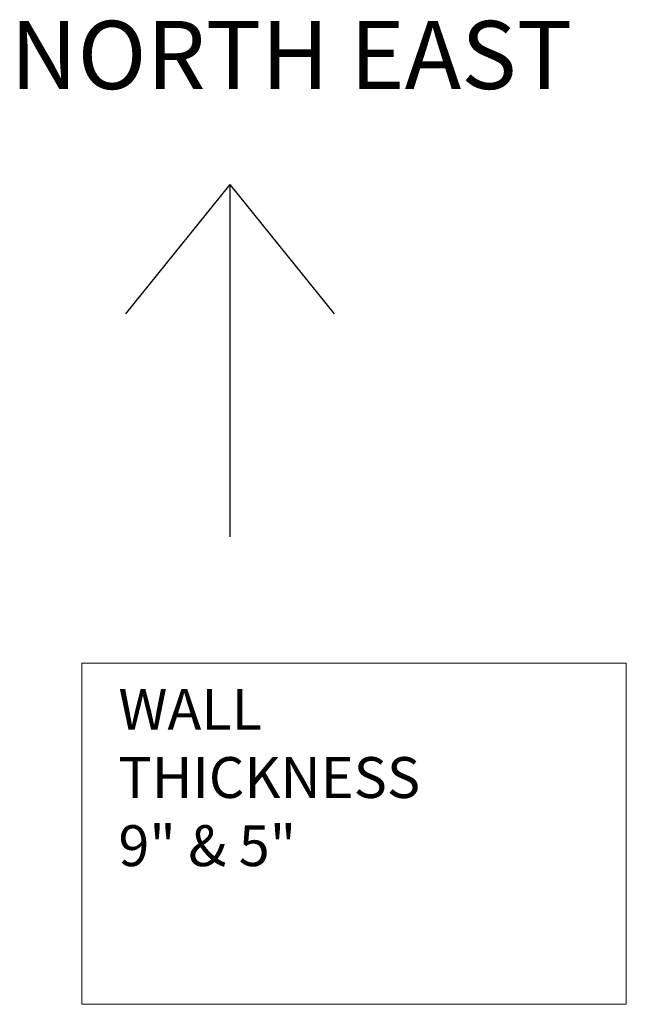
# Model space of a CAD drawing. Units: inches. Extents: x -2189 to 546, y 945 to 2684.
# Tile 10 of 10: x 13 to 546, y 1684 to 2551. Entities that reach past the tile are written whole.
import ezdxf

# ---------------------------------------------------------------- set-up
doc = ezdxf.new("R2010")
doc.units = ezdxf.units.IN
doc.header["$MEASUREMENT"] = 0
doc.layers.add('A-ANNO-SYMB', color=7, linetype='Continuous', lineweight=25)
doc.layers.add('A-ANNO-TEXT', color=7, linetype='Continuous', lineweight=18)
doc.styles.get("Standard").update_dxf_attribs({"font": 'arial.ttf'})

msp = doc.modelspace()

# ---------------------------------------------------------------- linework, layer by layer
at = {"layer": 'A-ANNO-SYMB'}
for q in [(105.65, 2291.59), (197.55, 2095.33), (289.46, 2291.59)]:
    msp.add_line((197.55, 2405.55), q, dxfattribs=at)
at = {"layer": 'A-ANNO-TEXT'}
msp.add_lwpolyline([(67.28, 1983.91), (546.47, 1983.91), (546.47, 1683.53), (67.28, 1683.53)], close=True, dxfattribs=at)

# ---------------------------------------------------------------- texts
at = {"layer": 'A-ANNO-SYMB', "insert": (4.33, 2549.69), "char_height": 60, "attachment_point": 1}
msp.add_mtext_dynamic_manual_height_columns('NORTH EAST', width=605.795, gutter_width=1, heights=[0], dxfattribs=at)
at = {"layer": 'A-ANNO-TEXT', "insert": (99.46, 1961.28), "char_height": 36, "attachment_point": 1}
msp.add_mtext_dynamic_manual_height_columns('WALL THICKNESS 9" & 5"', width=260.8599, gutter_width=1, heights=[0], dxfattribs=at)

doc.saveas('drawing.dxf')
